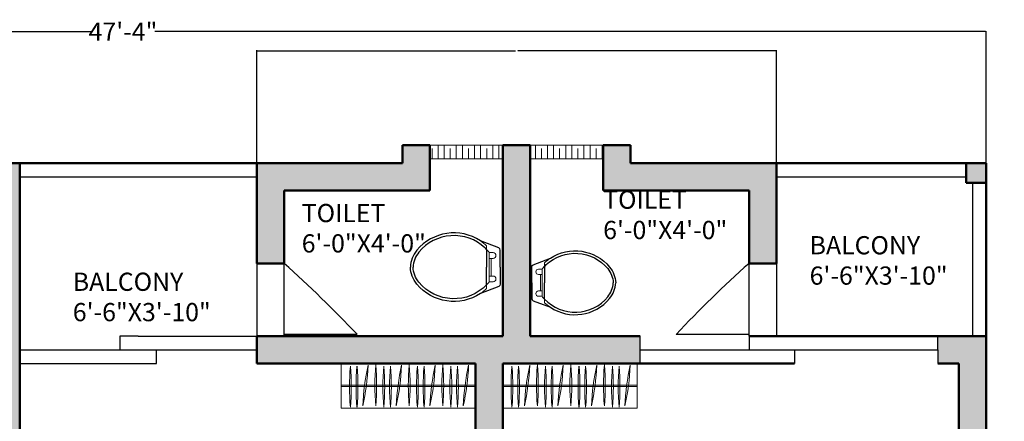
# Model space of a CAD drawing. Units: inches. Extents: x -12 to 604, y -566 to 58.
# Tile 12 of 12: x 280 to 604, y -74 to 58. Entities that reach past the tile are written whole.
import ezdxf

# ---------------------------------------------------------------- set-up
doc = ezdxf.new("R2010")
doc.units = ezdxf.units.IN
doc.header["$MEASUREMENT"] = 0
for name, color, linetype, lineweight in [('A-ANNO-DIMS', 2, 'Continuous', 18), ('A-AREA-IDEN', 7, 'Continuous', 18), ('A-DOOR', 4, 'Continuous', 25), ('A-FLOR-RAIL', 7, 'Continuous', 25), ('A-FURN', 8, 'Continuous', 18), ('A-GLAZ', 82, 'Continuous', 18), ('A-GLAZ-PATT', 82, 'Continuous', 13), ('A-WALL', 7, 'Continuous', 50), ('A-WALL-PATT', 18, 'Continuous', 13), ('WC-Detail_dwgmodels.com', 251, 'Continuous', 13), ('WC-Outline_dwgmodels.com', 250, 'Continuous', 25)]:
    doc.layers.add(name, color=color, linetype=linetype, lineweight=lineweight)
doc.styles.get("Standard").update_dxf_attribs({"font": 'arial.ttf'})
doc.dimstyles.get("Standard").update_dxf_attribs({"dimtxt": 0.18, "dimasz": 0.18, "dimexe": 0.18, "dimexo": 0.0625, "dimgap": 0.09, "dimtad": 0, "dimtih": 1, "dimtoh": 1, "dimdec": 0, "dimzin": 0, "dimdsep": 46, "dimlunit": 3, "dimtxsty": 'Standard', "dimcen": 0.09, "dimadec": 0, "dimazin": 0, "dimtfac": 1, "dimtdec": 0, "dimtofl": 0, "dimtmove": 0, "dimatfit": 3, "dimfxl": 1, "dimtolj": 1, "dimtzin": 0, "dimarcsym": 0})

# ---------------------------------------------------------------- blocks, each defined once
blk = doc.blocks.new('*D4')
at = {"layer": 'A-ANNO-DIMS', "color": 0, "lineweight": -2, "transparency": 16777216}
for p, q in [((30.32, 11.2), (30.32, 54.68)), ((30.5, 54.5), (303.81, 54.5)), ((598.14, 54.5), (324.84, 54.5)), ((598.32, 11.2), (598.32, 54.68))]:
    blk.add_line(p, q, dxfattribs=at)
at = {"layer": 'A-ANNO-DIMS', "color": 0, "transparency": 16777216}
for points in [[(30.5, 54.53), (30.5, 54.47), (30.32, 54.5)], [(598.14, 54.53), (598.14, 54.47), (598.32, 54.5)]]:
    blk.add_solid(points, dxfattribs=at)
at = {"layer": 'Defpoints', "color": 0, "transparency": 16777216}
for p in [(598.32, 54.5), (30.32, 11.14), (598.32, 11.14)]:
    blk.add_point(p, dxfattribs=at)
at = {"layer": 'A-ANNO-DIMS', "color": 0, "transparency": 16777216, "insert": (314.32, 54.5), "char_height": 6, "attachment_point": 5}
blk.add_mtext('\\A1;47\'-4"', dxfattribs=at)
blk = doc.blocks.new('WARDROBE-HANGING-RAIL')
for p, q in [((44.18, 14.73), (0, 14.73)), ((0, 14.73), (0, 0)), ((44.18, 14.73), (44.18, 0)), ((44.18, 7.61), (0, 7.61)), ((44.18, 7.12), (0, 7.12)), ((44.18, 0), (0, 0))]:
    blk.add_line(p, q)
for centre, start, end in [((80.19, 7.07), 175.0028, 184.9972), ((-74.2, 7.07), 355.0028, 4.9972), ((82.37, 7.07), 175.0028, 184.9972), ((-72.01, 7.07), 355.0028, 4.9972), ((-68.57, 17.55), 347.508, 357.5023), ((84.5, -2.59), 167.508, 177.5023), ((88.54, 7.54), 175.0028, 184.9972), ((-65.84, 7.54), 355.0028, 4.9972), ((91.2, 7.07), 175.0028, 184.9972), ((-63.19, 7.07), 355.0028, 4.9972), ((93.38, 7.07), 175.0028, 184.9972), ((-61.01, 7.07), 355.0028, 4.9972), ((-57.56, 17.55), 347.508, 357.5023), ((95.51, -2.59), 167.508, 177.5023), ((99.55, 7.54), 175.0028, 184.9972), ((-54.83, 7.54), 355.0028, 4.9972), ((102.24, 7.07), 175.0028, 184.9972), ((-52.14, 7.07), 355.0028, 4.9972), ((104.43, 7.07), 175.0028, 184.9972), ((-49.96, 7.07), 355.0028, 4.9972), ((106.56, -2.59), 167.508, 177.5023), ((-46.51, 17.55), 347.508, 357.5023), ((110.6, 7.54), 175.0028, 184.9972), ((-43.79, 7.54), 355.0028, 4.9972), ((113.25, 7.07), 175.0028, 184.9972), ((-41.13, 7.07), 355.0028, 4.9972), ((115.43, 7.07), 175.0028, 184.9972), ((-38.95, 7.07), 355.0028, 4.9972), ((117.56, -2.59), 167.508, 177.5023), ((-35.5, 17.55), 347.508, 357.5023)]:
    blk.add_arc(centre, 77.49, start, end)
blk = doc.blocks.new('*D53')
at = {"layer": 'A-ANNO-DIMS', "color": 0, "lineweight": -2, "transparency": 16777216}
for p, q in [((358.32, 11.2), (358.32, 48.37)), ((358.5, 48.19), (443.43, 48.19)), ((529.14, 48.19), (444.21, 48.19)), ((529.32, 11.2), (529.32, 48.37))]:
    blk.add_line(p, q, dxfattribs=at)
at = {"layer": 'A-ANNO-DIMS', "color": 0, "transparency": 16777216}
for points in [[(358.5, 48.22), (358.5, 48.16), (358.32, 48.19)], [(529.14, 48.22), (529.14, 48.16), (529.32, 48.19)]]:
    blk.add_solid(points, dxfattribs=at)
at = {"layer": 'Defpoints', "color": 0, "transparency": 16777216}
for p in [(529.32, 48.19), (358.32, 11.14), (529.32, 11.14)]:
    blk.add_point(p, dxfattribs=at)
at = {"layer": 'A-ANNO-DIMS', "color": 0, "transparency": 16777216, "insert": (443.82, 48.19), "char_height": 0.18, "attachment_point": 5}
blk.add_mtext('\\A1;14\'-3"', dxfattribs=at)

msp = doc.modelspace()

# ---------------------------------------------------------------- hatches: boundary and pattern name
at = {"layer": 'A-GLAZ-PATT'}
h = msp.add_hatch(dxfattribs=at)
h.set_pattern_fill('GOST_WOOD', color=256)
h.set_pattern_definition([(90, (0, 0), (6, -4e-16), [10, -2]), (90, (2, -2), (6, -4e-16), [6, -1.5, 3, -1.5]), (90, (4, -5), (6, -4e-16), [10, -2])])
h.paths.add_polyline_path([(229.32, 17.14), (169.32, 17.14), (169.32, 14.14), (169.32, 12.64), (229.32, 12.64)])
h.paths.add_polyline_path([(439.32, 17.14), (415.32, 17.14), (415.32, 12.64), (439.32, 12.64)])
h.paths.add_polyline_path([(472.32, 17.14), (448.32, 17.14), (448.32, 12.64), (472.32, 12.64)])
at = {"layer": 'A-WALL-PATT'}
h = msp.add_hatch(color=256, dxfattribs=at)
h.dxf.hatch_style = 1
h.paths.add_polyline_path([(169.32, 11.14), (169.32, 17.14), (160.32, 17.14), (160.32, 11.14), (118.32, 11.14), (118.32, 6.64), (118.32, 2.14), (127.32, 2.14), (169.32, 2.14)])
h.paths.add_polyline_path([(127.32, -13.61), (118.32, -13.61), (118.32, -29.36), (34.82, -29.36), (24.32, -29.36), (24.32, -38.36), (39.32, -38.36), (118.32, -38.36), (118.32, -126.86), (127.32, -126.86), (127.32, -117.86)])
h.paths.add_polyline_path([(82.32, -92.36), (39.32, -92.36), (39.32, -56.22), (30.32, -56.22), (24.32, -56.22), (24.32, -65.22), (30.32, -65.22), (30.32, -113.36), (24.32, -113.36), (24.32, -122.36), (39.32, -122.36), (39.32, -101.36), (82.32, -101.36), (82.32, -96.86)], flags=17)
h.paths.add_polyline_path([(280.32, 11.14), (238.32, 11.14), (238.32, 17.14), (229.32, 17.14), (229.32, 12.64), (229.32, 11.14), (229.32, 2.14), (271.32, 2.14), (271.32, -117.86), (163.32, -117.86), (163.32, -126.86), (271.32, -126.86), (271.32, -189.86), (280.32, -189.86), (280.32, -180.86)])
h.paths.add_polyline_path([(415.32, 17.14), (406.32, 17.14), (406.32, 11.14), (358.32, 11.14), (358.32, -21.86), (367.32, -21.86), (367.32, 2.14), (415.32, 2.14)], flags=17)
h.paths.add_polyline_path([(484.55, -45.86), (448.32, -45.86), (448.32, 2.14), (448.32, 17.14), (439.32, 17.14), (439.32, 12.64), (439.32, 2.14), (439.32, -45.86), (367.32, -45.86), (358.32, -45.86), (358.32, -54.86), (430.32, -54.86), (430.32, -69.59), (430.32, -180.86), (318.82, -180.86), (318.82, -189.86), (318.82, -331.86), (327.82, -331.86), (327.82, -189.86), (439.32, -189.86), (439.32, -180.86), (439.32, -54.86), (483.5, -54.86), (484.55, -54.86)])
h.paths.add_polyline_path([(529.32, 11.14), (481.32, 11.14), (481.32, 17.14), (472.32, 17.14), (472.32, 12.64), (472.32, 2.14), (520.32, 2.14), (520.32, -21.86), (529.32, -21.86)])
h.paths.add_polyline_path([(598.32, -45.86), (582.42, -45.86), (582.42, -50.36), (582.42, -54.86), (589.32, -54.86), (589.32, -99.86), (598.32, -99.86), (604.32, -99.86), (604.32, -90.86), (598.32, -90.86)])
h.paths.add_polyline_path([(598.32, -168.86), (604.32, -168.86), (604.32, -159.86), (589.32, -159.86), (589.32, -180.86), (477.32, -180.86), (477.32, -189.86), (477.32, -259.86), (486.32, -259.86), (486.32, -189.86), (589.32, -189.86), (589.32, -204.86), (598.32, -204.86), (604.32, -204.86), (604.32, -195.86), (598.32, -195.86)])
h.paths.add_polyline_path([(598.32, -244.86), (604.32, -244.86), (604.32, -235.86), (598.32, -235.86), (589.32, -235.86), (589.32, -250.86), (522.32, -250.86), (522.32, -259.86), (589.32, -259.86), (589.32, -274.86), (598.32, -274.86), (604.32, -274.86), (604.32, -265.86), (598.32, -265.86)])
h.paths.add_polyline_path([(598.32, -333.28), (604.32, -333.28), (604.32, -324.28), (598.32, -324.28), (598.32, -321.87), (598.32, -318.28), (604.32, -318.28), (604.32, -309.28), (598.32, -309.28), (589.32, -309.28), (589.32, -341.95), (589.38, -341.95), (589.38, -363.16), (589.32, -381.86), (565.32, -381.86), (565.32, -390.86), (589.32, -390.86), (589.32, -450.86), (598.32, -450.86), (604.32, -450.86), (604.32, -441.86), (598.32, -441.86), (598.32, -390.86), (604.32, -390.86), (604.32, -381.86), (598.32, -381.86)])
h.paths.add_polyline_path([(541.32, -345.86), (424.32, -345.86), (424.32, -354.86), (532.32, -354.86), (532.32, -474.86), (463.39, -474.86), (463.39, -483.86), (553.32, -483.86), (553.32, -474.86), (541.32, -474.86), (541.32, -390.86), (541.32, -381.86)])
h.paths.add_polyline_path([(604.32, -474.86), (589.32, -474.86), (553.32, -474.86), (553.32, -483.86), (598.32, -483.86), (604.32, -483.86)])
h.paths.add_polyline_path([(388.32, -483.86), (388.32, -474.86), (388.32, -460.13), (388.32, -333.86), (388.32, -322.86), (379.32, -322.86), (379.32, -331.86), (379.32, -333.86), (379.32, -474.86), (379.32, -520.86), (344.32, -520.86), (344.32, -529.86), (379.32, -529.86), (388.32, -529.86)])
h.paths.add_polyline_path([(284.32, -520.86), (249.32, -520.86), (249.32, -474.86), (249.32, -368.36), (240.32, -368.36), (240.32, -474.86), (238.52, -474.86), (238.52, -483.86), (240.32, -483.86), (240.32, -529.86), (249.32, -529.86), (284.32, -529.86)])
h.paths.add_polyline_path([(178.82, -474.86), (158.91, -474.86), (158.91, -483.86), (162.32, -483.86), (178.82, -483.86)])
h.paths.add_polyline_path([(84.32, -474.86), (84.32, -366.86), (75.32, -366.86), (75.32, -474.86), (39.32, -474.86), (39.32, -453.86), (24.32, -453.86), (24.32, -462.86), (30.32, -462.86), (30.32, -483.86), (84.32, -483.86)])
h.paths.add_polyline_path([(39.32, -342.86), (75.32, -342.86), (84.32, -342.86), (179.67, -342.86), (179.67, -333.86), (39.32, -333.86), (39.32, -318.86), (24.32, -318.86), (24.32, -327.86), (30.32, -327.86), (30.32, -432.86), (24.32, -432.86), (24.32, -441.86), (30.32, -441.86), (39.32, -441.86)])
h.paths.add_polyline_path([(249.32, -252.86), (115.32, -252.86), (115.32, -225.86), (106.32, -225.86), (106.32, -252.86), (39.32, -252.86), (39.32, -237.86), (24.32, -237.86), (24.32, -246.86), (30.32, -246.86), (30.32, -267.86), (24.32, -267.86), (24.32, -276.86), (39.32, -276.86), (39.32, -261.86), (240.32, -261.86), (240.32, -331.86), (249.32, -331.86), (266.82, -331.86), (266.82, -322.86), (249.32, -322.86)])
h.paths.add_polyline_path([(127.32, -180.86), (39.32, -180.86), (24.32, -180.86), (24.32, -189.86), (39.32, -189.86), (127.32, -189.86)])
h.paths.add_polyline_path([(39.32, -159.86), (24.32, -159.86), (24.32, -168.86), (30.32, -168.86), (30.32, -180.86), (39.32, -180.86)])
h.paths.add_polyline_path([(470.51, -17.27), (512.48, -17.27), (512.48, 5.12), (470.51, 5.12)], flags=9)
h.paths.add_polyline_path([(484.21, -244.26), (526.45, -244.26), (526.45, -221.87), (484.21, -221.87)], flags=24)
h.paths.add_polyline_path([(36.91, -442.88), (83.54, -442.88), (83.54, -420.5), (36.91, -420.5)], flags=25)
h = msp.add_hatch(color=256, dxfattribs=at)
h.dxf.hatch_style = 1
h.paths.add_polyline_path([(598.32, 11.14), (591.82, 11.14), (591.82, 6.64), (593.82, 6.64), (593.82, 4.64), (598.32, 4.64)])
h.paths.add_polyline_path([(36.82, 6.64), (36.82, 11.14), (30.32, 11.14), (30.32, 4.64), (34.82, 4.64), (36.82, 4.64)])
h = msp.add_hatch(color=256, dxfattribs=at)
h.dxf.hatch_style = 1
h.paths.add_polyline_path([(598.32, 11.14), (591.82, 11.14), (591.82, 6.64), (591.82, 4.64), (593.82, 4.64), (598.32, 4.64)])

# ---------------------------------------------------------------- linework, layer by layer
at = {"layer": 'A-DOOR'}
for p, q in [((358.32, -21.86), (358.32, -45.86)), ((358.32, -21.86), (367.32, -21.86)), ((367.32, -45.86), (367.32, -21.86)), ((520.32, -45.86), (520.32, -21.86)), ((520.32, -21.86), (529.32, -21.86)), ((529.32, -21.86), (529.32, -45.86)), ((367.32, -45.2), (391.32, -45.2)), ((520.32, -45.24), (496.32, -45.24)), ((319.32, -45.86), (313.32, -45.86)), ((313.32, -45.86), (313.32, -50.36)), ((319.32, -45.86), (358.32, -45.86)), ((358.32, -45.86), (367.32, -45.86)), ((484.55, -54.86), (484.55, -45.86)), ((529.32, -45.86), (520.32, -45.86)), ((520.32, -45.86), (520.32, -50.36)), ((582.42, -50.36), (582.42, -45.86)), ((280.32, -50.36), (358.32, -50.36)), ((325.32, -54.86), (325.32, -50.36)), ((484.55, -50.36), (529.32, -50.36)), ((529.32, -50.36), (535.32, -50.36)), ((535.32, -50.36), (535.32, -54.86)), ((535.32, -50.36), (582.42, -50.36)), ((582.42, -50.36), (582.42, -54.86)), ((280.32, -54.86), (319.32, -54.86)), ((319.32, -54.86), (325.32, -54.86))]:
    msp.add_line(p, q, dxfattribs=at)
for centre, radius, start, end in [((92.58, -328.33), 411.59, 43.4631, 48.1251), ((779.08, -311.46), 388.37, 131.7807, 136.7256)]:
    msp.add_arc(centre, radius, start, end, dxfattribs=at)
at = {"layer": 'A-FLOR-RAIL'}
for p, q in [((280.32, 6.64), (358.32, 6.64)), ((529.32, 6.64), (591.82, 6.64)), ((593.82, 4.64), (593.82, -45.86))]:
    msp.add_line(p, q, dxfattribs=at)
at = {"layer": 'A-GLAZ'}
for p, q in [((415.32, 17.14), (439.32, 17.14)), ((415.32, 12.64), (415.32, 17.14)), ((439.32, 17.14), (439.32, 12.64)), ((448.32, 17.14), (472.32, 17.14)), ((448.32, 12.64), (448.32, 17.14)), ((472.32, 17.14), (472.32, 12.64)), ((439.32, 12.64), (415.32, 12.64)), ((472.32, 12.64), (448.32, 12.64))]:
    msp.add_line(p, q, dxfattribs=at)
at = {"layer": 'A-WALL'}
for p, q in [((406.32, 17.14), (415.32, 17.14)), ((406.32, 17.14), (406.32, 11.14)), ((415.32, 17.14), (415.32, 2.14)), ((439.32, 2.14), (439.32, 17.14)), ((439.32, 17.14), (448.32, 17.14)), ((448.32, 2.14), (448.32, 17.14)), ((472.32, 17.14), (472.32, 2.14)), ((472.32, 17.14), (481.32, 17.14)), ((481.32, 17.14), (481.32, 11.14)), ((238.32, 11.14), (406.32, 11.14)), ((280.32, 11.14), (280.32, -189.86)), ((358.32, 11.14), (358.32, -21.86)), ((481.32, 11.14), (598.32, 11.14)), ((529.32, 11.14), (529.32, -21.86)), ((591.82, 6.64), (591.82, 11.14)), ((598.32, 11.14), (598.32, -90.86)), ((591.82, 6.64), (591.82, 4.64)), ((591.82, 4.64), (593.82, 4.64)), ((593.82, 4.64), (598.32, 4.64)), ((367.32, 2.14), (367.32, -21.86)), ((367.32, 2.14), (415.32, 2.14)), ((439.32, 2.14), (439.32, -45.86)), ((448.32, 2.14), (448.32, -45.86)), ((472.32, 2.14), (520.32, 2.14)), ((520.32, 2.14), (520.32, -21.86)), ((367.32, -21.86), (358.32, -21.86)), ((520.32, -21.86), (529.32, -21.86)), ((358.32, -45.86), (367.32, -45.86)), ((358.32, -45.86), (358.32, -54.86)), ((367.32, -45.86), (439.32, -45.86)), ((448.32, -45.86), (484.55, -45.86)), ((529.32, -45.86), (520.32, -45.86)), ((529.32, -45.86), (598.32, -45.86)), ((358.32, -54.86), (430.32, -54.86)), ((430.32, -54.86), (430.32, -180.86)), ((439.32, -54.86), (439.32, -189.86)), ((439.32, -54.86), (535.32, -54.86)), ((582.42, -54.86), (589.32, -54.86)), ((589.32, -54.86), (589.32, -99.86))]:
    msp.add_line(p, q, dxfattribs=at)
at = {"layer": 'WC-Detail_dwgmodels.com'}
for p, q in [((433.97, -16.05), (433.97, -17.29)), ((453.05, -21.65), (453.05, -22.81)), ((433.97, -28.92), (433.97, -30.16)), ((453.05, -33.66), (453.05, -34.82))]:
    msp.add_line(p, q, dxfattribs=at)
for points in [[(433.97, -16.05, 0.040937), (431.94, -14.45, 0.163732)], [(434.86, -18.31, 0.022712), (433.97, -17.29, 0.162618)], [(434.86, -23.11), (434.86, -18.31, 0.022712)], [(434.86, -18.31), (436.1, -18.31, -1), (436.1, -20.2), (435.46, -20.2)], [(453.05, -21.65, -0.040937), (454.94, -20.16, -0.163732)], [(434.86, -23.11), (434.86, -27.91, -0.476108)], [(452.21, -23.76), (451.06, -23.76, 1), (451.06, -25.52), (451.66, -25.52)], [(452.21, -23.76, -0.022712), (453.05, -22.81, -0.162618)], [(452.21, -28.24), (452.21, -23.76, -0.022712)], [(434.86, -27.91, -0.022712), (433.97, -28.92, -0.162618)], [(434.86, -27.91), (436.1, -27.91, 1), (436.1, -26.02), (435.46, -26.02)], [(452.21, -28.24), (452.21, -32.71, 0.476108)], [(433.97, -30.16, -0.040937), (431.94, -31.77, -0.163732)], [(452.21, -32.71), (451.06, -32.71, -1), (451.06, -30.95), (451.66, -30.95)], [(452.21, -32.71, 0.022712), (453.05, -33.66, 0.162618)], [(453.05, -34.82, 0.040937), (454.94, -36.31, 0.163732)]]:
    msp.add_lwpolyline(points, format="xyb", dxfattribs=at)
for points in [[(435.46, -20.2), (434.86, -20.2)], [(435.46, -26.02), (435.46, -20.2)], [(451.66, -30.95), (451.66, -25.52)], [(451.66, -25.52), (452.21, -25.52)], [(435.46, -26.02), (434.86, -26.02)], [(451.66, -30.95), (452.21, -30.95)]]:
    msp.add_lwpolyline(points, dxfattribs=at)
at = {"layer": 'WC-Outline_dwgmodels.com'}
for p, q in [((433.97, -17.29), (433.97, -23.11)), ((433.97, -28.92), (433.97, -23.11)), ((453.05, -22.81), (453.05, -28.24)), ((453.05, -33.66), (453.05, -28.24))]:
    msp.add_line(p, q, dxfattribs=at)
for points in [[(431.94, -14.45, 0.383919), (411.02, -17.55, 0.163732), (408.89, -23.11, 0.359733)], [(433.37, -16.7, 0.431639), (411.7, -18.12, 0.162618), (409.77, -23.11, 0.470877)], [(438.45, -23.11), (438.45, -17.46, 0.31031), (437.97, -16.77), (431.94, -14.45, 0.209071)], [(433.97, -17.29, 0.014165), (433.37, -16.7, 0.162618)], [(453.61, -22.26, -0.431639), (473.83, -23.58, -0.162618), (475.62, -28.24, -0.470877)], [(454.94, -20.16, -0.383919), (474.46, -23.05, -0.163732), (476.45, -28.24, -0.359733)], [(448.87, -28.24), (448.87, -22.97, -0.31031), (449.31, -22.32), (454.94, -20.16, -0.209071)], [(453.05, -22.81, -0.014165), (453.61, -22.26, -0.162618)], [(431.94, -31.77, -0.383919), (411.02, -28.67, -0.163732), (408.89, -23.11, -0.359733)], [(433.97, -28.92, -0.448546), (411.7, -28.1, -0.162618), (409.77, -23.11, -0.470877)], [(438.45, -23.11), (438.45, -28.75, -0.31031), (437.97, -29.45), (431.94, -31.77, -0.209071)], [(448.87, -28.24), (448.87, -33.5, 0.31031), (449.31, -34.15), (454.94, -36.31, 0.209071)], [(453.05, -33.66, 0.448546), (473.83, -32.89, 0.162618), (475.62, -28.24, 0.470877)], [(454.94, -36.31, 0.383919), (474.46, -33.42, 0.163732), (476.45, -28.24, 0.359733)]]:
    msp.add_lwpolyline(points, format="xyb", dxfattribs=at)

# ---------------------------------------------------------------- block references
at = {"layer": 'A-FURN'}
for p in [(386.14, -69.59), (439.32, -69.59)]:
    msp.add_blockref('WARDROBE-HANGING-RAIL', p, dxfattribs=at)

# ---------------------------------------------------------------- texts
at = {"layer": 'A-AREA-IDEN', "insert": (472.32, 2.14), "char_height": 6, "attachment_point": 1}
msp.add_mtext_dynamic_manual_height_columns('TOILET\\P6\'-0"X4\'-0"', width=0.2503, gutter_width=1, heights=[0], dxfattribs=at)
at = {"layer": 'A-AREA-IDEN', "char_height": 6, "attachment_point": 1}
for s, insert in [('TOILET\\P6\'-0"X4\'-0"', (373.13, -2.27)), ('BALCONY\\P6\'-6"X3\'-10"', (540.27, -12.88)), ('BALCONY\\P6\'-6"X3\'-10"', (297.8, -24.91))]:
    msp.add_mtext(s, dxfattribs=dict(at, insert=insert))

# ---------------------------------------------------------------- dimensions: what is measured, and where the dimension line sits
at = {"layer": 'A-ANNO-DIMS'}
for base, p1, p2, override, picture, middle in [((598.32, 54.5), (30.32, 11.14), (598.32, 11.14), {"dimtxt": 6, "dimclrd": 0, "dimclre": 0, "dimclrt": 0}, '*D4', (314.32, 54.5)), ((529.32, 48.19), (358.32, 11.14), (529.32, 11.14), {"dimdec": 1, "dimlfac": 1, "dimrnd": 0, "dimzin": 1, "dimdsep": 46, "dimlunit": 4, "dimfrac": 2}, '*D53', (443.82, 48.19))]:
    dim = msp.add_linear_dim(base=base, p1=p1, p2=p2, dimstyle='Standard', override=override, dxfattribs=at)
    dim.commit()
    dim.dimension.update_dxf_attribs({"geometry": picture, "text_midpoint": middle})

doc.saveas('drawing.dxf')
